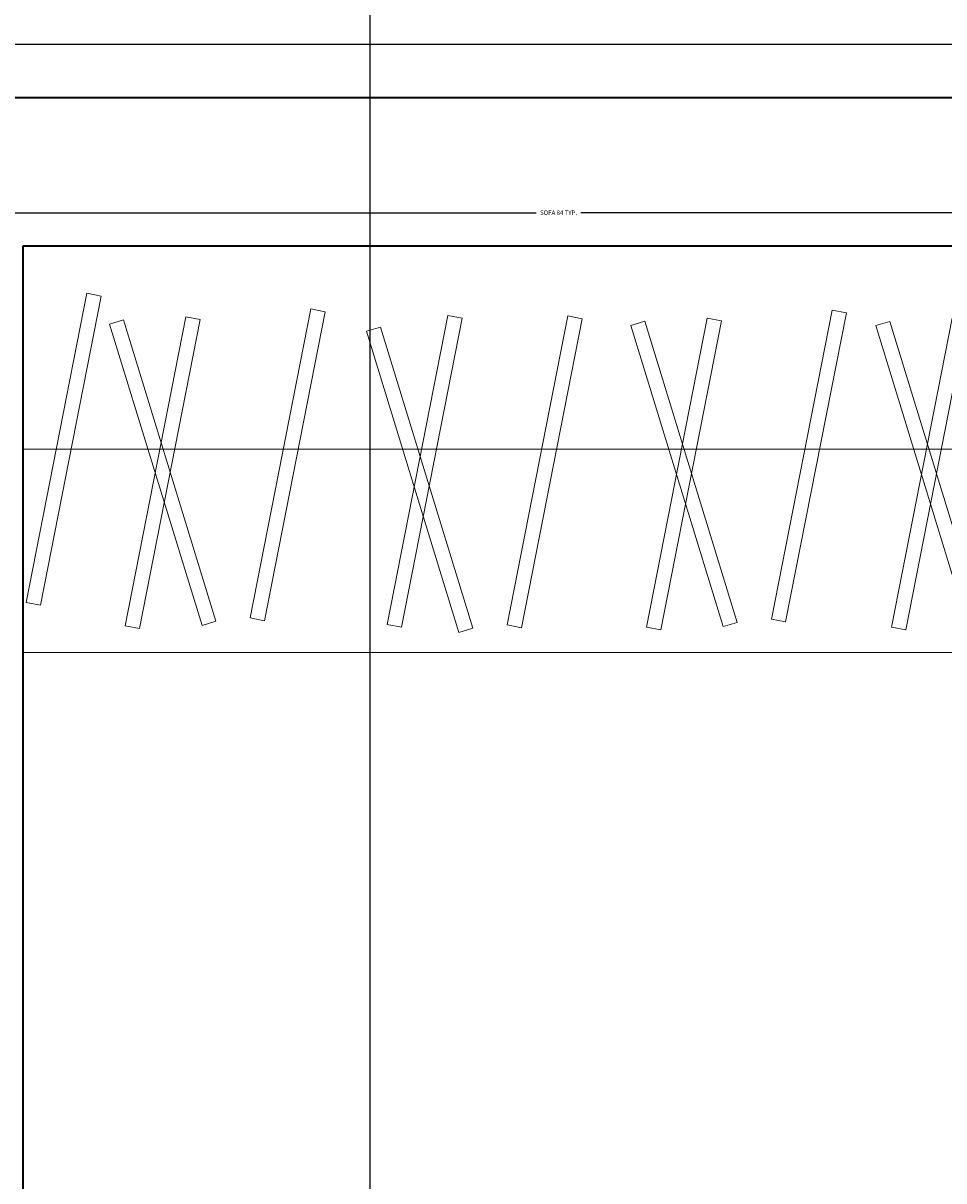
# Model space of a CAD drawing. Units: inches. Extents: x -61 to 1599, y -1316 to 257.
# Tile 65 of 204: x 166 to 203, y -213 to -166. Entities that reach past the tile are written whole.
import ezdxf

# ---------------------------------------------------------------- set-up
doc = ezdxf.new("R2010")
doc.units = ezdxf.units.IN
doc.header["$MEASUREMENT"] = 0
for name, color, linetype, lineweight in [('A-ANNO-DIMS', 2, 'Continuous', 18), ('A-FLOR-CASE', 8, 'Continuous', 18), ('WALLS', 4, 'Continuous', 35)]:
    doc.layers.add(name, color=color, linetype=linetype, lineweight=lineweight)
doc.styles.get("Standard").update_dxf_attribs({"font": 'arial.ttf'})
doc.dimstyles.get("Standard").update_dxf_attribs({"dimtxt": 0.18, "dimasz": 0.18, "dimexe": 0.18, "dimexo": 0.0625, "dimgap": 0.09, "dimtad": 0, "dimtih": 1, "dimtoh": 1, "dimdec": 0, "dimzin": 0, "dimdsep": 46, "dimlunit": 3, "dimtxsty": 'Standard', "dimcen": 0.09, "dimadec": 0, "dimazin": 0, "dimtfac": 1, "dimtdec": 0, "dimtofl": 0, "dimtmove": 0, "dimatfit": 3, "dimfxl": 1, "dimtolj": 1, "dimtzin": 0, "dimarcsym": 0})

# ---------------------------------------------------------------- blocks, each defined once
blk = doc.blocks.new('WARDROBE-HANGING-2')
blk.add_line((55.703, 8.23), (0, 8.23))
for points in [[(55.703, 16.46), (55.703, 0), (0, 0), (0, 16.46)], [(0.121, 2.033), (2.581, 14.541), (3.16, 14.427), (0.7, 1.92)], [(44.491, 1.561), (46.952, 14.069), (47.53, 13.955), (45.07, 1.448)], [(49.548, 1.88), (52.008, 14.387), (52.587, 14.273), (50.127, 1.766)], [(54.096, 14.328), (54.096, 1.581), (53.506, 1.581), (53.506, 14.328)], [(4.131, 1.085), (6.591, 13.592), (7.17, 13.478), (4.709, 0.971)], [(9.187, 1.403), (11.648, 13.911), (12.226, 13.797), (9.766, 1.289)], [(14.733, 1.142), (17.193, 13.649), (17.772, 13.535), (15.312, 1.028)], [(19.586, 1.118), (22.047, 13.625), (22.625, 13.511), (20.165, 1.004)], [(30.284, 1.352), (32.745, 13.859), (33.323, 13.745), (30.863, 1.238)], [(40.204, 1.348), (42.664, 13.855), (43.243, 13.742), (40.782, 1.234)], [(47.6, 1.579), (43.858, 13.764), (44.421, 13.937), (48.164, 1.752)], [(7.24, 1.102), (3.497, 13.288), (4.061, 13.461), (7.804, 1.276)], [(17.639, 0.817), (13.896, 13.002), (14.46, 13.175), (18.203, 0.99)], [(28.337, 1.051), (24.594, 13.236), (25.158, 13.409), (28.901, 1.224)], [(25.228, 1.034), (27.688, 13.541), (28.267, 13.427), (25.806, 0.92)], [(38.256, 1.047), (34.513, 13.232), (35.077, 13.406), (38.82, 1.221)], [(35.147, 1.03), (37.607, 13.537), (38.186, 13.423), (35.726, 0.916)]]:
    blk.add_lwpolyline(points, close=True)
blk = doc.blocks.new('*D670')
at = {"layer": 'A-ANNO-DIMS', "color": 0, "lineweight": -2, "transparency": 16777216}
for p, q in [((145.375, -161.442), (145.375, -174.159)), ((229.375, -161.442), (229.375, -174.159)), ((145.555, -173.979), (186.47, -173.979)), ((229.195, -173.979), (188.279, -173.979))]:
    blk.add_line(p, q, dxfattribs=at)
at = {"layer": 'A-ANNO-DIMS', "color": 0, "transparency": 16777216}
for points in [[(145.555, -173.949), (145.555, -174.009), (145.375, -173.979)], [(229.195, -173.949), (229.195, -174.009), (229.375, -173.979)]]:
    blk.add_solid(points, dxfattribs=at)
at = {"layer": 'DEFPOINTS', "color": 0, "transparency": 16777216}
for p in [(145.375, -161.379), (229.375, -161.379), (229.375, -173.979)]:
    blk.add_point(p, dxfattribs=at)
at = {"layer": 'A-ANNO-DIMS', "color": 0, "transparency": 16777216, "insert": (187.375, -173.979), "char_height": 0.18, "attachment_point": 5}
blk.add_mtext('\\A1;SOFA 84 TYP.', dxfattribs=at)
blk = doc.blocks.new('*D687')
at = {"layer": 'A-ANNO-DIMS', "color": 0, "lineweight": -2, "transparency": 16777216}
for p, q in [((289.418, 181.677), (-61.077, 181.677)), ((-60.897, 181.497), (-60.897, -528.952)), ((-60.897, -1239.765), (-60.897, -529.316)), ((319.64, -1239.945), (-61.077, -1239.945))]:
    blk.add_line(p, q, dxfattribs=at)
at = {"layer": 'A-ANNO-DIMS', "color": 0, "transparency": 16777216}
for points in [[(-60.927, 181.497), (-60.867, 181.497), (-60.897, 181.677)], [(-60.927, -1239.765), (-60.867, -1239.765), (-60.897, -1239.945)]]:
    blk.add_solid(points, dxfattribs=at)
at = {"layer": 'DEFPOINTS', "color": 0, "transparency": 16777216}
for p in [(289.481, 181.677), (-60.897, -1239.945), (319.703, -1239.945)]:
    blk.add_point(p, dxfattribs=at)
at = {"layer": 'A-ANNO-DIMS', "color": 0, "transparency": 16777216, "insert": (-60.897, -529.134), "char_height": 0.18, "attachment_point": 5}
blk.add_mtext('\\A1;1421.6', dxfattribs=at)
blk = doc.blocks.new('*D699')
at = {"layer": 'A-ANNO-DIMS', "color": 0, "lineweight": -2, "transparency": 16777216}
for p, q in [((835.64, -167.169), (-61.077, -167.169)), ((-60.897, -167.349), (-60.897, -306.726)), ((-60.897, -446.466), (-60.897, -307.09)), ((841.64, -446.646), (-61.077, -446.646))]:
    blk.add_line(p, q, dxfattribs=at)
at = {"layer": 'A-ANNO-DIMS', "color": 0, "transparency": 16777216}
for points in [[(-60.927, -167.349), (-60.867, -167.349), (-60.897, -167.169)], [(-60.927, -446.466), (-60.867, -446.466), (-60.897, -446.646)]]:
    blk.add_solid(points, dxfattribs=at)
at = {"layer": 'DEFPOINTS', "color": 0, "transparency": 16777216}
for p in [(835.703, -167.169), (-60.897, -446.646), (841.703, -446.646)]:
    blk.add_point(p, dxfattribs=at)
at = {"layer": 'A-ANNO-DIMS', "color": 0, "transparency": 16777216, "insert": (-60.897, -306.908), "char_height": 0.18, "attachment_point": 5}
blk.add_mtext('\\A1;279.5', dxfattribs=at)
blk = doc.blocks.new('*D700')
at = {"layer": 'A-ANNO-DIMS', "color": 0, "lineweight": -2, "transparency": 16777216}
for p, q in [((14.703, -616.882), (14.703, 257.457)), ((14.883, 257.277), (96.772, 257.277)), ((179.572, 257.277), (97.683, 257.277)), ((179.752, -616.882), (179.752, 257.457))]:
    blk.add_line(p, q, dxfattribs=at)
at = {"layer": 'A-ANNO-DIMS', "color": 0, "transparency": 16777216}
for points in [[(14.883, 257.307), (14.883, 257.247), (14.703, 257.277)], [(179.572, 257.307), (179.572, 257.247), (179.752, 257.277)]]:
    blk.add_solid(points, dxfattribs=at)
at = {"layer": 'DEFPOINTS', "color": 0, "transparency": 16777216}
for p in [(179.752, 257.277), (14.703, -616.945), (179.752, -616.945)]:
    blk.add_point(p, dxfattribs=at)
at = {"layer": 'A-ANNO-DIMS', "color": 0, "transparency": 16777216, "insert": (97.227, 257.277), "char_height": 0.18, "attachment_point": 5}
blk.add_mtext('\\A1;165.05', dxfattribs=at)

msp = doc.modelspace()

# ---------------------------------------------------------------- linework, layer by layer
at = {"layer": 'WALLS'}
for p, q in [((119.7028, -169.3229), (234.7028, -169.3229)), ((165.7028, -282.3229), (165.7028, -175.3229)), ((165.7028, -175.3229), (228.7028, -175.3229))]:
    msp.add_line(p, q, dxfattribs=at)

# ---------------------------------------------------------------- block references
at = {"layer": 'A-FLOR-CASE'}
msp.add_blockref('WARDROBE-HANGING-2', (165.703, -191.783), dxfattribs=at)

# ---------------------------------------------------------------- dimensions: what is measured, and where the dimension line sits
at = {"layer": 'A-ANNO-DIMS'}
dim = msp.add_linear_dim(base=(179.7521, 257.2771), p1=(14.7028, -616.9446), p2=(179.7521, -616.9446), dimstyle='Standard', override={"dimdec": 2, "dimlfac": 1, "dimrnd": 0, "dimzin": 0, "dimdsep": 46, "dimlunit": 2}, dxfattribs=at)
dim.commit()
dim.dimension.update_dxf_attribs({"geometry": '*D700', "text_midpoint": (97.2274, 257.2771)})
for base, p1, p2, picture, middle in [((-60.8972, -1239.9446), (289.4807, 181.6771), (319.7028, -1239.9446), '*D687', (-60.8972, -529.1337)), ((-60.8972, -446.6462), (835.7028, -167.169), (841.7028, -446.6462), '*D699', (-60.8972, -306.9076))]:
    dim = msp.add_linear_dim(base=base, p1=p1, p2=p2, angle=90, dimstyle='Standard', override={"dimdec": 1, "dimlfac": 1, "dimrnd": 0, "dimzin": 0, "dimdsep": 46, "dimlunit": 2}, dxfattribs=at)
    dim.commit()
    dim.dimension.update_dxf_attribs({"geometry": picture, "text_midpoint": middle})
dim = msp.add_linear_dim(base=(229.3746, -173.9792), p1=(145.3746, -161.3792), p2=(229.3746, -161.3792), text='SOFA <> TYP.', dimstyle='Standard', override={"dimdec": 0, "dimlfac": 1, "dimrnd": 0, "dimzin": 0, "dimdsep": 46, "dimlunit": 2}, dxfattribs=at)
dim.commit()
dim.dimension.update_dxf_attribs({"geometry": '*D670', "text_midpoint": (187.3746, -173.9792)})

doc.saveas('drawing.dxf')
